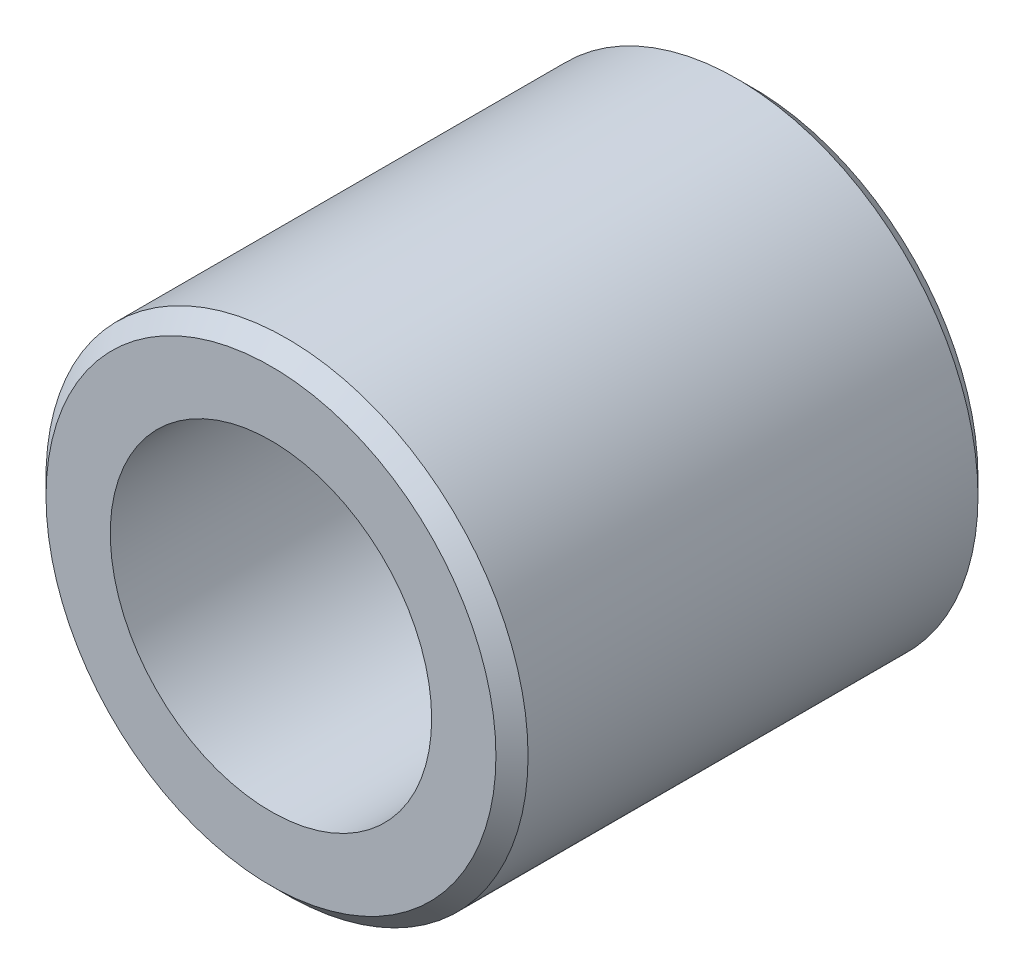
SolidWorks part; units mm, degrees
material "Plain Carbon Steel"
ref_plane "Front Plane" through (0, 0, 0) normal (0, 0, 1) x (1, 0, 0)
ref_plane "Top Plane" through (0, 0, 0) normal (0, 1, 0) x (1, 0, 0)
ref_plane "Right Plane" through (0, 0, 0) normal (1, 0, 0) x (0, 0, -1)
sketch "Bushing Profile Ø30-Ø20" plane through (0, 0, 0) normal (0, 0, 1) x (1, 0, 0)
  circle A0 centre (0, 0) radius 10
  circle A1 centre (0, 0) radius 15
  dimension "D1" = 20
  dimension "D2" = 30
extrude "Bushing Body L30" add sketch "Bushing Profile Ø30-Ø20" along normal mid plane 30
chamfer "Outer Edge Chamfers 1x45°" distance 1 angle 45 2 edges at (15, 0, -15) (15, 0, 15)
